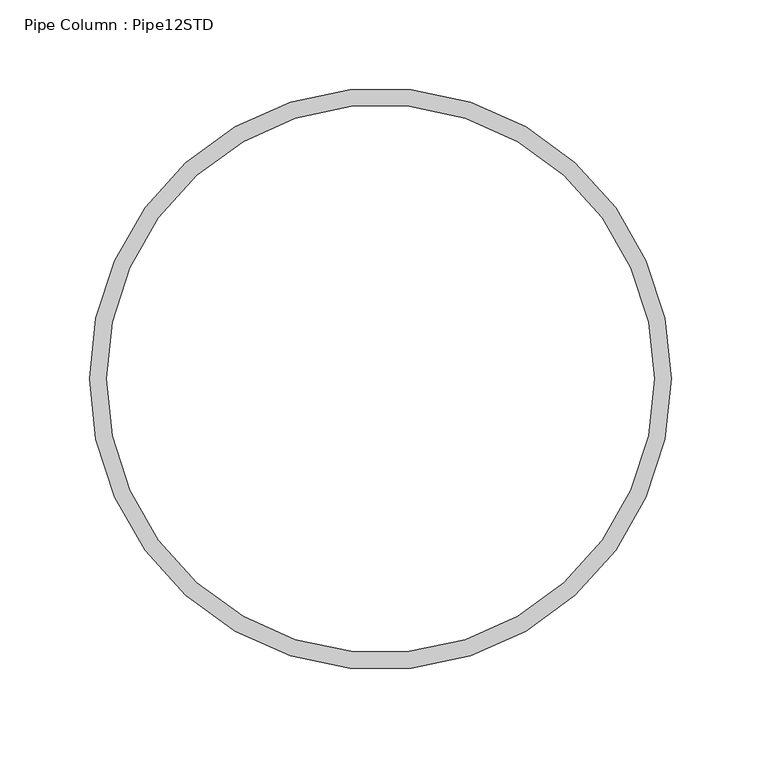
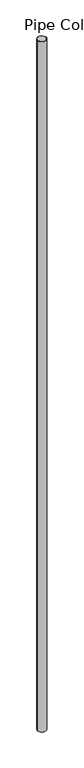
"""IFC4 building model written with IfcOpenShell, lengths in millimetres: column geometry, Pipe Column : Pipe12STD."""

from ifc_helpers import new_model, si_unit, point, origin, origin_with_axes, origin_2d, place, context, project, spatial, circle_curve, trimmed, segment, composite_curve, outline, extrude, source, transform, mapped, element, save


def pipe_column_pipe12std_f9386f83(model_context):
    return source(origin(), model_context, "Body", "SweptSolid", [
        extrude(outline(composite_curve([segment(trimmed(circle_curve(origin_2d(), 162.56), [point((-162.56, 0.0))], [point((162.56, 0.0))], False, "CARTESIAN"), True, "CONTINUOUS"), segment(trimmed(circle_curve(origin_2d(), 162.56), [point((162.56, 0.0))], [point((-162.56, 0.0))], False, "CARTESIAN"), True, "CONTINUOUS")], self_intersect=False), holes=[composite_curve([segment(trimmed(circle_curve(origin_2d(), 153.035), [point((-153.035, 0.0))], [point((153.035, 0.0))], True, "CARTESIAN"), True, "CONTINUOUS"), segment(trimmed(circle_curve(origin_2d(), 153.035), [point((153.035, 0.0))], [point((-153.035, 0.0))], True, "CARTESIAN"), True, "CONTINUOUS")], self_intersect=False)]), origin_with_axes(), (0.0, 0.0, 1.0), 27000.0),
    ])


if __name__ == "__main__":
    model = new_model("IFC4")
    model_context = context("Model", 3, world=origin())
    ifc_project = project(units=[si_unit("LENGTHUNIT", "METRE", prefix="MILLI")], contexts=[model_context])
    site = spatial("IfcSite", under=ifc_project)
    building = spatial("IfcBuilding", under=site)
    placement = place(None, origin())
    pipe_column_pipe12std_shape = pipe_column_pipe12std_f9386f83(model_context)
    element("IfcColumn", 1, ObjectType="Pipe Column : Pipe12STD", at=placement, inside=building, context=model_context, shape_type="MappedRepresentation", body=[
        mapped(pipe_column_pipe12std_shape, transform((0.0, 0.0, 0.0), x_axis=(1.0, 0.0, 0.0), y_axis=(0.0, 1.0, 0.0), z_axis=(0.0, 0.0, 1.0))),
    ])
    save(model, "model.ifc")

# Revit data of these elements
# Type "Pipe Column : Pipe12STD"
#   Section Name Key = "Pipe 12 Std"
#   Assembly Code = "B10"
#   Wall Nominal Thickness = 0.9525 cm
#   Wall Design Thickness = 0.8865 cm
#   Torsional Moment of Inertia = 21768.90 cm⁴
#   Section Area = 88.3869 cm²
#   Plastic Modulus weak axis = 879.985 cm³
#   Plastic Modulus strong axis = 879.985 cm³
#   Nominal Weight = 73.8129 kgf/m
#   Moment of Inertia weak axis = 10905.26 cm⁴
#   Moment of Inertia strong axis = 10905.26 cm⁴
#   Elastic Modulus weak axis = 671.87 cm³
#   Elastic Modulus strong axis = 671.87 cm³
#   Diameter = 32.512 cm
#   Centroid Vertical = 16.256 cm
#   Centroid Horizontal = 16.256 cm
#   Structural Material [instance default] = Steel ASTM A53
#   Warping Constant = (empty or 0)
#   Torsional Modulus = 0
#   Principal Axes Angle = 0
# Element 1 (IfcColumn, "Pipe Column : Pipe12STD")
#   Materials on its faces: "Steel ASTM A53"
# Materials
#   "Steel ASTM A53": class "Metal", colour RGB 199 199 199, transparency 0, Description = "Carbon steel", Cost = 0
